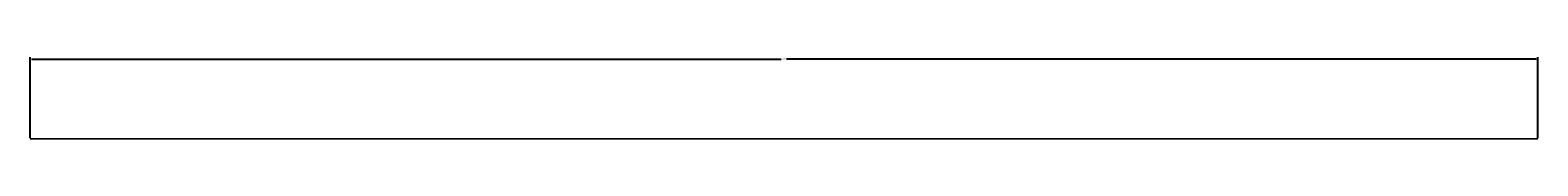
# Model space of a CAD drawing. Units: millimetres. Extents: x 392 to 548, y 0 to 8.
import ezdxf

# ---------------------------------------------------------------- set-up
doc = ezdxf.new("R2010")
doc.units = ezdxf.units.MM
doc.layers.add('M-CONS', color=5, linetype='Continuous', lineweight=18)
doc.layers.add('M-DIMS', color=2, linetype='Continuous', lineweight=18)
doc.styles.get("Standard").update_dxf_attribs({"font": 'arial.ttf'})
doc.dimstyles.get("Standard").update_dxf_attribs({"dimtxt": 0.18, "dimasz": 0.18, "dimexe": 0.18, "dimexo": 0.0625, "dimgap": 0.09, "dimtad": 0, "dimtih": 1, "dimtoh": 1, "dimdec": 4, "dimzin": 0, "dimdsep": 46, "dimtxsty": 'Standard', "dimcen": 0.09, "dimadec": 0, "dimazin": 0, "dimtfac": 1, "dimtdec": 4, "dimtofl": 0, "dimtmove": 0, "dimatfit": 3, "dimfxl": 1, "dimtolj": 1, "dimtzin": 0, "dimarcsym": 0})

# ---------------------------------------------------------------- blocks, each defined once
blk = doc.blocks.new('*D1')
at = {"layer": 'Defpoints', "color": 0, "transparency": 16777216}
for p in [(548.46, 8.25), (392.46, 0), (548.46, 0)]:
    blk.add_point(p, dxfattribs=at)
at = {"layer": 'M-DIMS', "color": 0, "lineweight": -2, "transparency": 16777216}
for p, q in [((392.46, 0.06), (392.46, 8.43)), ((392.64, 8.25), (470.18, 8.25)), ((548.28, 8.25), (470.74, 8.25)), ((548.46, 0.06), (548.46, 8.43))]:
    blk.add_line(p, q, dxfattribs=at)
at = {"layer": 'M-DIMS', "color": 0, "transparency": 16777216}
for points in [[(392.64, 8.28), (392.64, 8.22), (392.46, 8.25)], [(548.28, 8.28), (548.28, 8.22), (548.46, 8.25)]]:
    blk.add_solid(points, dxfattribs=at)
at = {"layer": 'M-DIMS', "color": 0, "transparency": 16777216, "insert": (470.46, 8.25), "char_height": 0.18, "attachment_point": 5}
blk.add_mtext('\\A1;156', dxfattribs=at)

msp = doc.modelspace()

# ---------------------------------------------------------------- linework, layer by layer
at = {"layer": 'M-CONS', "extrusion": (0, -1, 0)}
msp.add_lwpolyline([(426.46, 174.27), (426.46, 169.85, -7.364208), (418.46, 169.85), (418.46, 174.27), (422.46, 174.27)], format="xyb", close=True, dxfattribs=at)
for points in [[(511.64, 169.2, 0.511352), (508.71, 181.83, 0.142312), (449.4, 188.67, 0.590785), (444.79, 175.43)], [(452.16, 159.69, 0.459755), (462.41, 153.18, -0.131289), (497.49, 154.43, 0.410497), (507.06, 160.34)]]:
    msp.add_lwpolyline(points, format="xyb", dxfattribs=at)
for centre, radius in [((422.46, 155.39), 30), ((527.46, 155.39), 21), ((527.46, 155.39), 10)]:
    msp.add_circle(centre, radius, dxfattribs=at)
for centre, radius, start, end in [((467.29, 83.17), 115, 50.1991, 121.8296), ((482.29, 88.15), 60, 56.105, 131.6641)]:
    msp.add_arc(centre, radius, start, end, dxfattribs=at)

# ---------------------------------------------------------------- dimensions: what is measured, and where the dimension line sits
at = {"layer": 'M-DIMS'}
dim = msp.add_linear_dim(base=(548.46, 8.25), p1=(392.46, 0), p2=(548.46, 0), dimstyle='Standard', override={"dimdec": 0, "dimlfac": 1, "dimrnd": 0, "dimzin": 0, "dimdsep": 46, "dimlunit": 2}, dxfattribs=at)
dim.commit()
dim.dimension.update_dxf_attribs({"geometry": '*D1', "text_midpoint": (470.46, 8.25)})

doc.saveas('drawing.dxf')
